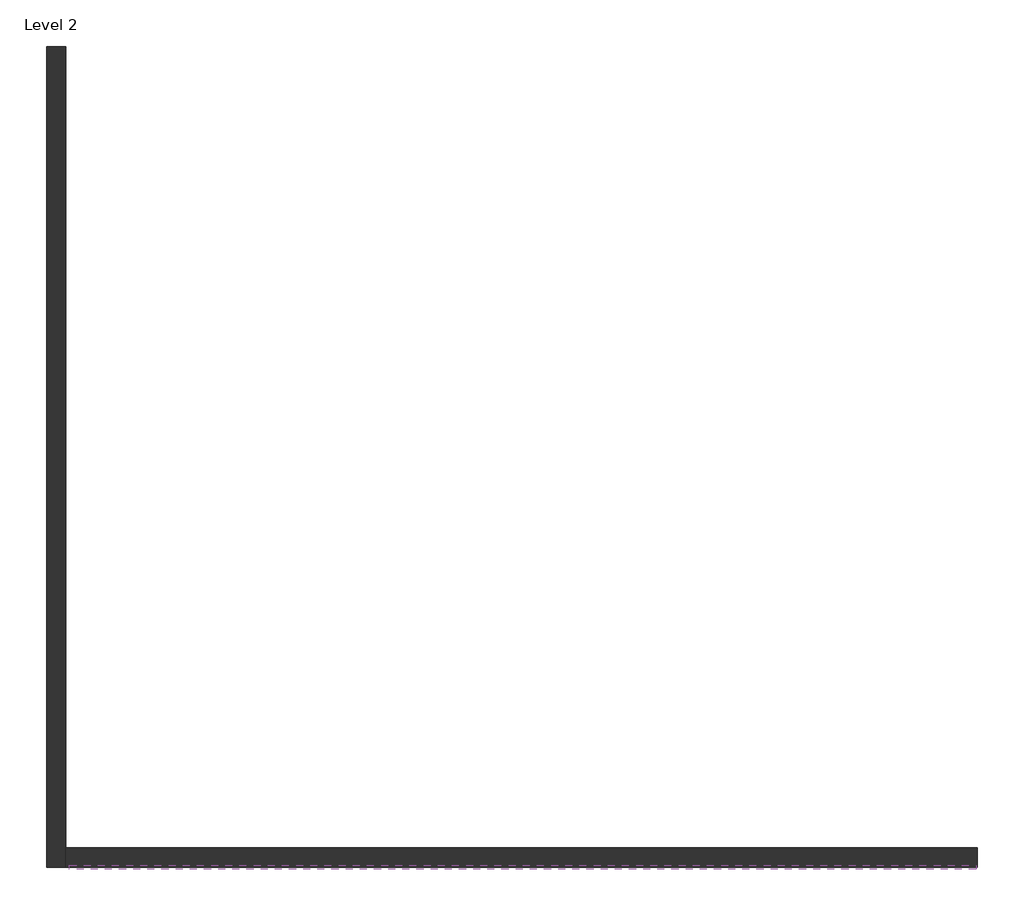
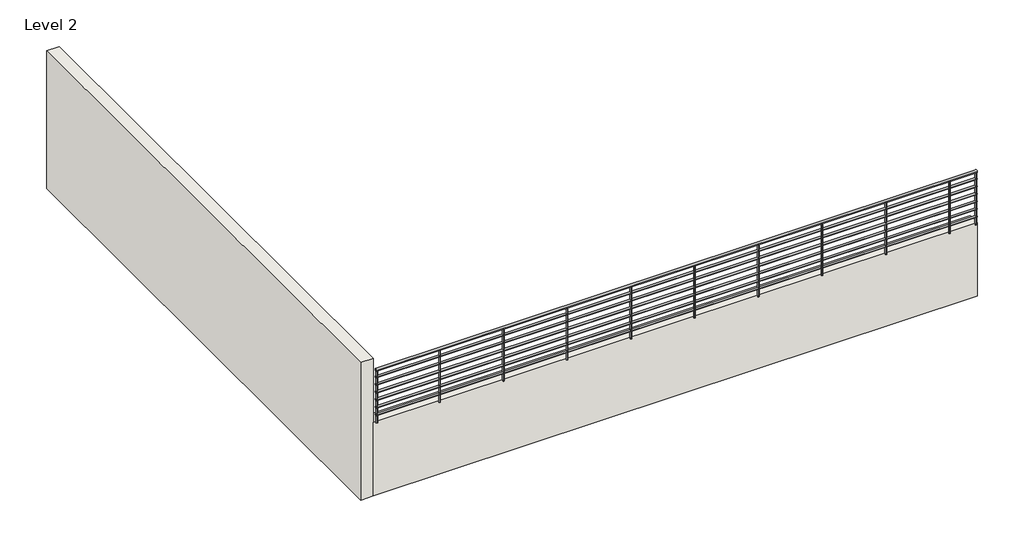
# One storey: 2 walls, 1 railing.
"""IFC4 building model written with IfcOpenShell, lengths in millimetres."""

from ifc_helpers import new_model, si_unit, point, frame, frame_2d, origin, place, context, project, spatial, polyline, circle_curve, trimmed, segment, composite_curve, outline, extrude, faceted_brep, element, save

model = new_model("IFC4")

# Units and contexts
model_context = context("Model", 3, world=origin())
ifc_project = project(units=[si_unit("LENGTHUNIT", "METRE", prefix="MILLI")], contexts=[model_context])

# Site, building, storey
site = spatial("IfcSite", under=ifc_project)
building = spatial("IfcBuilding", under=site)
storey = spatial("IfcBuildingStorey", under=building, Name="Level 2", Elevation=6096.0)

# Railing
placement = place(None, origin())
element("IfcRailing", 1, ObjectType="900mm Pipe", at=placement, inside=storey, context=model_context, shape_type="SweptSolid", body=[
    extrude(outline(composite_curve([segment(trimmed(circle_curve(frame_2d((-798.6874979, 8176.9243707)), 20.0), [point((-818.6874979, 8176.9243707))], [point((-778.6874979, 8176.9243707))], False, "CARTESIAN"), True, "CONTINUOUS"), segment(trimmed(circle_curve(frame_2d((-798.6874979, 8176.9243707)), 20.0), [point((-778.6874979, 8176.9243707))], [point((-818.6874979, 8176.9243707))], False, "CARTESIAN"), True, "CONTINUOUS")], self_intersect=False)), frame((-2887.6371352, 0.0, 0.0), z_axis=(1.0, 0.0, 0.0), x_axis=(0.0, 1.0, 0.0)), (0.0, 0.0, 1.0), 9423.4),
    extrude(outline(composite_curve([segment(trimmed(circle_curve(frame_2d((-798.6874979, 8056.9243707)), 15.0), [point((-783.6874979, 8056.9243707))], [point((-813.6874979, 8056.9243707))], False, "CARTESIAN"), True, "CONTINUOUS"), segment(trimmed(circle_curve(frame_2d((-798.6874979, 8056.9243707)), 15.0), [point((-813.6874979, 8056.9243707))], [point((-783.6874979, 8056.9243707))], False, "CARTESIAN"), True, "CONTINUOUS")], self_intersect=False)), frame((-2887.6371352, 0.0, 0.0), z_axis=(1.0, 0.0, 0.0), x_axis=(0.0, 1.0, 0.0)), (0.0, 0.0, 1.0), 9423.4),
    extrude(outline(composite_curve([segment(trimmed(circle_curve(frame_2d((-798.6874979, 7931.9243707)), 15.0), [point((-783.6874979, 7931.9243707))], [point((-813.6874979, 7931.9243707))], False, "CARTESIAN"), True, "CONTINUOUS"), segment(trimmed(circle_curve(frame_2d((-798.6874979, 7931.9243707)), 15.0), [point((-813.6874979, 7931.9243707))], [point((-783.6874979, 7931.9243707))], False, "CARTESIAN"), True, "CONTINUOUS")], self_intersect=False)), frame((-2887.6371352, 0.0, 0.0), z_axis=(1.0, 0.0, 0.0), x_axis=(0.0, 1.0, 0.0)), (0.0, 0.0, 1.0), 9423.4),
    extrude(outline(composite_curve([segment(trimmed(circle_curve(frame_2d((-798.6874979, 7806.9243707)), 15.0), [point((-783.6874979, 7806.9243707))], [point((-813.6874979, 7806.9243707))], False, "CARTESIAN"), True, "CONTINUOUS"), segment(trimmed(circle_curve(frame_2d((-798.6874979, 7806.9243707)), 15.0), [point((-813.6874979, 7806.9243707))], [point((-783.6874979, 7806.9243707))], False, "CARTESIAN"), True, "CONTINUOUS")], self_intersect=False)), frame((-2887.6371352, 0.0, 0.0), z_axis=(1.0, 0.0, 0.0), x_axis=(0.0, 1.0, 0.0)), (0.0, 0.0, 1.0), 9423.4),
    extrude(outline(composite_curve([segment(trimmed(circle_curve(frame_2d((-798.6874979, 7681.9243707)), 15.0), [point((-783.6874979, 7681.9243707))], [point((-813.6874979, 7681.9243707))], False, "CARTESIAN"), True, "CONTINUOUS"), segment(trimmed(circle_curve(frame_2d((-798.6874979, 7681.9243707)), 15.0), [point((-813.6874979, 7681.9243707))], [point((-783.6874979, 7681.9243707))], False, "CARTESIAN"), True, "CONTINUOUS")], self_intersect=False)), frame((-2887.6371352, 0.0, 0.0), z_axis=(1.0, 0.0, 0.0), x_axis=(0.0, 1.0, 0.0)), (0.0, 0.0, 1.0), 9423.4),
    extrude(outline(composite_curve([segment(trimmed(circle_curve(frame_2d((-798.6874979, 7556.9243707)), 15.0), [point((-783.6874979, 7556.9243707))], [point((-813.6874979, 7556.9243707))], False, "CARTESIAN"), True, "CONTINUOUS"), segment(trimmed(circle_curve(frame_2d((-798.6874979, 7556.9243707)), 15.0), [point((-813.6874979, 7556.9243707))], [point((-783.6874979, 7556.9243707))], False, "CARTESIAN"), True, "CONTINUOUS")], self_intersect=False)), frame((-2887.6371352, 0.0, 0.0), z_axis=(1.0, 0.0, 0.0), x_axis=(0.0, 1.0, 0.0)), (0.0, 0.0, 1.0), 9423.4),
    extrude(outline(composite_curve([segment(trimmed(circle_curve(frame_2d((-798.6874979, 7431.9243707)), 15.0), [point((-783.6874979, 7431.9243707))], [point((-813.6874979, 7431.9243707))], False, "CARTESIAN"), True, "CONTINUOUS"), segment(trimmed(circle_curve(frame_2d((-798.6874979, 7431.9243707)), 15.0), [point((-813.6874979, 7431.9243707))], [point((-783.6874979, 7431.9243707))], False, "CARTESIAN"), True, "CONTINUOUS")], self_intersect=False)), frame((-2887.6371352, 0.0, 0.0), z_axis=(1.0, 0.0, 0.0), x_axis=(0.0, 1.0, 0.0)), (0.0, 0.0, 1.0), 9423.4),
    extrude(outline(composite_curve([segment(trimmed(circle_curve(frame_2d((6112.3628648, -798.6874979)), 12.5), [point((6112.3628648, -786.1874979))], [point((6112.3628648, -811.1874979))], False, "CARTESIAN"), True, "CONTINUOUS"), segment(trimmed(circle_curve(frame_2d((6112.3628648, -798.6874979)), 12.5), [point((6112.3628648, -811.1874979))], [point((6112.3628648, -786.1874979))], False, "CARTESIAN"), True, "CONTINUOUS")], self_intersect=False)), frame((0.0, 0.0, 7296.9243707), z_axis=(0.0, 0.0, 1.0), x_axis=(1.0, 0.0, 0.0)), (0.0, 0.0, 1.0), 860.0),
    extrude(outline(composite_curve([segment(trimmed(circle_curve(frame_2d((5112.3628648, -798.6874979)), 12.5), [point((5112.3628648, -786.1874979))], [point((5112.3628648, -811.1874979))], False, "CARTESIAN"), True, "CONTINUOUS"), segment(trimmed(circle_curve(frame_2d((5112.3628648, -798.6874979)), 12.5), [point((5112.3628648, -811.1874979))], [point((5112.3628648, -786.1874979))], False, "CARTESIAN"), True, "CONTINUOUS")], self_intersect=False)), frame((0.0, 0.0, 7296.9243707), z_axis=(0.0, 0.0, 1.0), x_axis=(1.0, 0.0, 0.0)), (0.0, 0.0, 1.0), 860.0),
    extrude(outline(composite_curve([segment(trimmed(circle_curve(frame_2d((4112.3628648, -798.6874979)), 12.5), [point((4112.3628648, -786.1874979))], [point((4112.3628648, -811.1874979))], False, "CARTESIAN"), True, "CONTINUOUS"), segment(trimmed(circle_curve(frame_2d((4112.3628648, -798.6874979)), 12.5), [point((4112.3628648, -811.1874979))], [point((4112.3628648, -786.1874979))], False, "CARTESIAN"), True, "CONTINUOUS")], self_intersect=False)), frame((0.0, 0.0, 7296.9243707), z_axis=(0.0, 0.0, 1.0), x_axis=(1.0, 0.0, 0.0)), (0.0, 0.0, 1.0), 860.0),
    extrude(outline(composite_curve([segment(trimmed(circle_curve(frame_2d((3112.3628648, -798.6874979)), 12.5), [point((3112.3628648, -786.1874979))], [point((3112.3628648, -811.1874979))], False, "CARTESIAN"), True, "CONTINUOUS"), segment(trimmed(circle_curve(frame_2d((3112.3628648, -798.6874979)), 12.5), [point((3112.3628648, -811.1874979))], [point((3112.3628648, -786.1874979))], False, "CARTESIAN"), True, "CONTINUOUS")], self_intersect=False)), frame((0.0, 0.0, 7296.9243707), z_axis=(0.0, 0.0, 1.0), x_axis=(1.0, 0.0, 0.0)), (0.0, 0.0, 1.0), 860.0),
    extrude(outline(composite_curve([segment(trimmed(circle_curve(frame_2d((2112.3628648, -798.6874979)), 12.5), [point((2112.3628648, -786.1874979))], [point((2112.3628648, -811.1874979))], False, "CARTESIAN"), True, "CONTINUOUS"), segment(trimmed(circle_curve(frame_2d((2112.3628648, -798.6874979)), 12.5), [point((2112.3628648, -811.1874979))], [point((2112.3628648, -786.1874979))], False, "CARTESIAN"), True, "CONTINUOUS")], self_intersect=False)), frame((0.0, 0.0, 7296.9243707), z_axis=(0.0, 0.0, 1.0), x_axis=(1.0, 0.0, 0.0)), (0.0, 0.0, 1.0), 860.0),
    extrude(outline(composite_curve([segment(trimmed(circle_curve(frame_2d((1112.3628648, -798.6874979)), 12.5), [point((1112.3628648, -786.1874979))], [point((1112.3628648, -811.1874979))], False, "CARTESIAN"), True, "CONTINUOUS"), segment(trimmed(circle_curve(frame_2d((1112.3628648, -798.6874979)), 12.5), [point((1112.3628648, -811.1874979))], [point((1112.3628648, -786.1874979))], False, "CARTESIAN"), True, "CONTINUOUS")], self_intersect=False)), frame((0.0, 0.0, 7296.9243707), z_axis=(0.0, 0.0, 1.0), x_axis=(1.0, 0.0, 0.0)), (0.0, 0.0, 1.0), 860.0),
    extrude(outline(composite_curve([segment(trimmed(circle_curve(frame_2d((112.3628648, -798.6874979)), 12.5), [point((112.3628648, -786.1874979))], [point((112.3628648, -811.1874979))], False, "CARTESIAN"), True, "CONTINUOUS"), segment(trimmed(circle_curve(frame_2d((112.3628648, -798.6874979)), 12.5), [point((112.3628648, -811.1874979))], [point((112.3628648, -786.1874979))], False, "CARTESIAN"), True, "CONTINUOUS")], self_intersect=False)), frame((0.0, 0.0, 7296.9243707), z_axis=(0.0, 0.0, 1.0), x_axis=(1.0, 0.0, 0.0)), (0.0, 0.0, 1.0), 860.0),
    extrude(outline(composite_curve([segment(trimmed(circle_curve(frame_2d((-887.6371352, -798.6874979)), 12.5), [point((-887.6371352, -786.1874979))], [point((-887.6371352, -811.1874979))], False, "CARTESIAN"), True, "CONTINUOUS"), segment(trimmed(circle_curve(frame_2d((-887.6371352, -798.6874979)), 12.5), [point((-887.6371352, -811.1874979))], [point((-887.6371352, -786.1874979))], False, "CARTESIAN"), True, "CONTINUOUS")], self_intersect=False)), frame((0.0, 0.0, 7296.9243707), z_axis=(0.0, 0.0, 1.0), x_axis=(1.0, 0.0, 0.0)), (0.0, 0.0, 1.0), 860.0),
    extrude(outline(composite_curve([segment(trimmed(circle_curve(frame_2d((-1887.6371352, -798.6874979)), 12.5), [point((-1887.6371352, -786.1874979))], [point((-1887.6371352, -811.1874979))], False, "CARTESIAN"), True, "CONTINUOUS"), segment(trimmed(circle_curve(frame_2d((-1887.6371352, -798.6874979)), 12.5), [point((-1887.6371352, -811.1874979))], [point((-1887.6371352, -786.1874979))], False, "CARTESIAN"), True, "CONTINUOUS")], self_intersect=False)), frame((0.0, 0.0, 7296.9243707), z_axis=(0.0, 0.0, 1.0), x_axis=(1.0, 0.0, 0.0)), (0.0, 0.0, 1.0), 860.0),
    extrude(outline(composite_curve([segment(trimmed(circle_curve(frame_2d((6523.2628648, -798.6874979)), 12.5), [point((6523.2628648, -786.1874979))], [point((6523.2628648, -811.1874979))], False, "CARTESIAN"), True, "CONTINUOUS"), segment(trimmed(circle_curve(frame_2d((6523.2628648, -798.6874979)), 12.5), [point((6523.2628648, -811.1874979))], [point((6523.2628648, -786.1874979))], False, "CARTESIAN"), True, "CONTINUOUS")], self_intersect=False)), frame((0.0, 0.0, 7296.9243707), z_axis=(0.0, 0.0, 1.0), x_axis=(1.0, 0.0, 0.0)), (0.0, 0.0, 1.0), 860.0),
    extrude(outline(composite_curve([segment(trimmed(circle_curve(frame_2d((-2875.1371352, -798.6874979)), 12.5), [point((-2875.1371352, -786.1874979))], [point((-2875.1371352, -811.1874979))], False, "CARTESIAN"), True, "CONTINUOUS"), segment(trimmed(circle_curve(frame_2d((-2875.1371352, -798.6874979)), 12.5), [point((-2875.1371352, -811.1874979))], [point((-2875.1371352, -786.1874979))], False, "CARTESIAN"), True, "CONTINUOUS")], self_intersect=False)), frame((0.0, 0.0, 7296.9243707), z_axis=(0.0, 0.0, 1.0), x_axis=(1.0, 0.0, 0.0)), (0.0, 0.0, 1.0), 860.0),
])

# Walls
element("IfcWall", 2, ObjectType="Generic - 9\"", at=placement, inside=storey, context=model_context, shape_type="Brep", body=[
    faceted_brep([(-3125.3625081, 7735.7125021, 6096.0), (-3125.3625081, -798.6874979, 6096.0), (-3125.3625081, -798.6874979, 8382.0), (-3125.3625081, 7735.7125021, 8382.0), (-2925.3625081, 7735.7125021, 6096.0), (-2925.3625081, 7735.7125021, 8382.0), (-2925.3625081, -798.6874979, 8382.0), (-2925.3625081, -798.6874979, 7315.2), (-2925.3625081, -798.6874979, 6096.0), (-2925.3625081, -598.6874979, 6096.0)], [[[0, 1, 2, 3]], [[4, 5, 6, 7, 8, 9]], [[1, 0, 4, 9, 8]], [[3, 2, 6, 5]], [[0, 3, 5, 4]], [[2, 1, 8, 7, 6]]]),
])
element("IfcWall", 3, ObjectType="Generic - 9\"", at=placement, inside=storey, context=model_context, shape_type="SweptSolid", body=[
    extrude(outline(polyline([(-2925.3625081, -598.6874979), (6550.4374919, -598.6874979), (6550.4374919, -798.6874979), (-2925.3625081, -798.6874979), (-2925.3625081, -598.6874979)])), frame((0.0, 0.0, 6096.0), z_axis=(0.0, 0.0, 1.0), x_axis=(1.0, 0.0, 0.0)), (0.0, 0.0, 1.0), 1219.2),
])

save(model, "model.ifc")

# Revit data of these elements
# Type "900mm Pipe"
#   built-in parameter 1008612 = 0.019685 (stored number, unit not read)
#   built-in parameter 1008611 = 0.0984252 (stored number, unit not read)
#   built-in parameter 1008609 = 6.56168 (stored number, unit not read)
#   built-in parameter 1008604 = 0.19685 (stored number, unit not read)
#   built-in parameter 1008603 = 0.164042 (stored number, unit not read)
#   Railing Height = 2' - 11.43307"
#   built-in parameter 1008630 = 2
#   built-in parameter 1008610 = 2
#   built-in parameter 1008605 = 1
#   built-in parameter 1008618 = M_Baluster - Round : 25mm
# Type "Generic - 9\""
#   Layers, outside or top first: 0' - 7.87402" no material (function 1)
# Element 1 (IfcRailing, "900mm Pipe")
#   built-in parameter 1008621 = 3.94004 (stored number, unit not read)
#   Phase Created = New Construction
# Element 2 (IfcWall, "Generic - 9\"")
#   Top Offset = 0' - 0"
#   Base Offset = 0' - 0"
#   Unconnected Height = 7' - 6"
#   wall height = 7' - 6"
#   Phase Created = New Construction
#   Base Constraint = Level 2
#   Materials on its faces: "Default Wall"
# Element 3 (IfcWall, "Generic - 9\"")
#   Top Offset = 0' - 0"
#   Base Offset = 0' - 0"
#   Unconnected Height = 4' - 0"
#   wall height = 4' - 0"
#   Phase Created = New Construction
#   Base Constraint = Level 2
#   Materials on its faces: "Default Wall"
# Materials
#   "Default Wall": colour RGB 80 80 80, transparency 0
